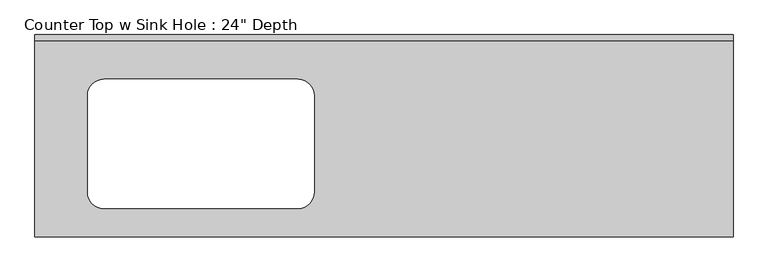
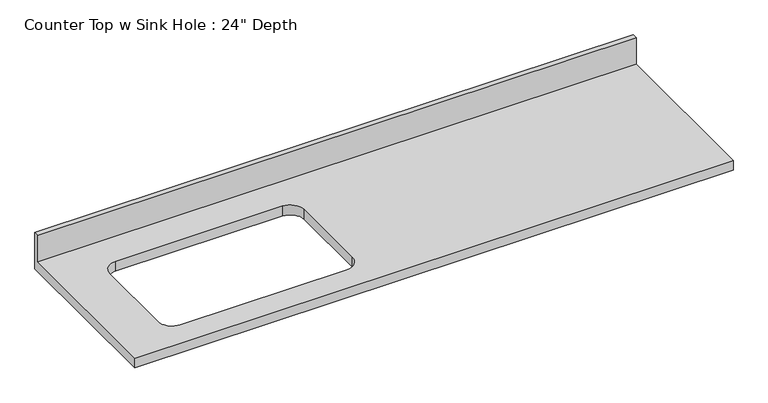
"""IFC4 building model written with IfcOpenShell, lengths in millimetres: furniture geometry."""

from ifc_helpers import new_model, si_unit, frame, origin, place, context, project, spatial, polyline, circle_curve, source, transform, mapped, element, save
from ifc_brep_helpers import plane_surface, revolved_surface, advanced_brep


def furniture_74614b7d(model_context):
    return source(origin(), model_context, "Body", "AdvancedBrep", [
        advanced_brep(
        [(-1200.4622951, -635.0, 914.4), (990.2877049, -635.0, 914.4), (990.2877049, -19.05, 914.4), (-1200.4622951, -19.05, 914.4), (-984.5622951, -139.7, 914.4), (-374.9622951, -139.7, 914.4), (-324.1622951, -190.5, 914.4), (-324.1622951, -495.3, 914.4), (-374.9622951, -546.1, 914.4), (-984.5622951, -546.1, 914.4), (-1035.3622951, -495.3, 914.4), (-1035.3622951, -190.5, 914.4), (990.2877049, 0.0, 876.3), (990.2877049, -635.0, 876.3), (-1200.4622951, -635.0, 876.3), (-1200.4622951, 0.0, 876.3), (-374.9622951, -139.7, 876.3), (-984.5622951, -139.7, 876.3), (-1035.3622951, -190.5, 876.3), (-1035.3622951, -495.3, 876.3), (-984.5622951, -546.1, 876.3), (-374.9622951, -546.1, 876.3), (-324.1622951, -495.3, 876.3), (-324.1622951, -190.5, 876.3), (-1200.4622951, 0.0, 1016.0), (990.2877049, 0.0, 1016.0), (-1200.4622951, -19.05, 1016.0), (990.2877049, -19.05, 1016.0)],
        [
            (0, 1),
            (1, 2),
            (2, 3),
            (3, 0),
            (4, 5),
            (5, 6, circle_curve(frame((-374.9622951, -190.5, 914.4), z_axis=(0.0, 0.0, -1.0), x_axis=(1.0, 0.0, 0.0)), 50.8)),
            (6, 7),
            (7, 8, circle_curve(frame((-374.9622951, -495.3, 914.4), z_axis=(0.0, 0.0, -1.0), x_axis=(1.0, 0.0, 0.0)), 50.8)),
            (8, 9),
            (9, 10, circle_curve(frame((-984.5622951, -495.3, 914.4), z_axis=(0.0, 0.0, -1.0), x_axis=(1.0, 0.0, 0.0)), 50.8)),
            (10, 11),
            (11, 4, circle_curve(frame((-984.5622951, -190.5, 914.4), z_axis=(0.0, 0.0, -1.0), x_axis=(1.0, 0.0, 0.0)), 50.8)),
            (12, 13),
            (13, 14),
            (14, 15),
            (15, 12),
            (16, 17),
            (17, 18, circle_curve(frame((-984.5622951, -190.5, 876.3), z_axis=(0.0, 0.0, 1.0), x_axis=(1.0, 0.0, 0.0)), 50.8)),
            (18, 19),
            (19, 20, circle_curve(frame((-984.5622951, -495.3, 876.3), z_axis=(0.0, 0.0, 1.0), x_axis=(1.0, 0.0, 0.0)), 50.8)),
            (20, 21),
            (21, 22, circle_curve(frame((-374.9622951, -495.3, 876.3), z_axis=(0.0, 0.0, 1.0), x_axis=(1.0, 0.0, 0.0)), 50.8)),
            (22, 23),
            (23, 16, circle_curve(frame((-374.9622951, -190.5, 876.3), z_axis=(0.0, 0.0, 1.0), x_axis=(1.0, 0.0, 0.0)), 50.8)),
            (15, 24),
            (24, 25),
            (25, 12),
            (14, 0),
            (3, 26),
            (26, 24),
            (13, 1),
            (25, 27),
            (27, 2),
            (26, 27),
            (4, 17),
            (16, 5),
            (11, 18),
            (10, 19),
            (9, 20),
            (8, 21),
            (7, 22),
            (6, 23),
        ],
        [
            plane_surface(frame((-1200.4622951, 0.0, 914.4), z_axis=(0.0, 0.0, 1.0), x_axis=(-1.0, 0.0, 0.0))),
            plane_surface(frame((-1200.4622951, 0.0, 876.3), z_axis=(0.0, 0.0, -1.0), x_axis=(1.0, 0.0, 0.0))),
            plane_surface(frame((990.2877049, 0.0, 914.4), z_axis=(0.0, 1.0, 0.0), x_axis=(0.0, 0.0, -1.0))),
            plane_surface(frame((-1200.4622951, 0.0, 914.4), z_axis=(-1.0, 0.0, 0.0), x_axis=(0.0, 0.0, -1.0))),
            plane_surface(frame((-1200.4622951, -635.0, 914.4), z_axis=(0.0, -1.0, 0.0), x_axis=(0.0, 0.0, -1.0))),
            plane_surface(frame((990.2877049, -635.0, 914.4), z_axis=(1.0, 0.0, 0.0), x_axis=(0.0, 0.0, -1.0))),
            plane_surface(frame((-1200.4622951, 0.0, 1016.0), z_axis=(0.0, 0.0, 1.0), x_axis=(0.0, -1.0, 0.0))),
            plane_surface(frame((-1200.4622951, -19.05, 1016.0), z_axis=(0.0, -1.0, 0.0), x_axis=(0.0, 0.0, -1.0))),
            plane_surface(frame((-374.9622951, -139.7, 914.4), z_axis=(0.0, -1.0, 0.0), x_axis=(0.0, 0.0, -1.0))),
            revolved_surface(polyline([(-933.7622951000001, -190.5, 914.4), (-933.7622951000001, -190.5, 876.3)]), (-984.5622951, -190.5, 876.3), (0.0, 0.0, 1.0)),
            plane_surface(frame((-1035.3622951, -190.5, 914.4), z_axis=(1.0, 0.0, 0.0), x_axis=(0.0, 0.0, -1.0))),
            revolved_surface(polyline([(-933.7622951000001, -495.3, 914.4), (-933.7622951000001, -495.3, 876.3)]), (-984.5622951, -495.3, 876.3), (0.0, 0.0, 1.0)),
            plane_surface(frame((-984.5622951, -546.1, 914.4), z_axis=(0.0, 1.0, 0.0), x_axis=(0.0, 0.0, -1.0))),
            revolved_surface(polyline([(-324.1622951, -495.3, 914.4), (-324.1622951, -495.3, 876.3)]), (-374.9622951, -495.3, 876.3), (0.0, 0.0, 1.0)),
            plane_surface(frame((-324.1622951, -495.3, 914.4), z_axis=(-1.0, 0.0, 0.0), x_axis=(0.0, 0.0, -1.0))),
            revolved_surface(polyline([(-324.1622951, -190.5, 914.4), (-324.1622951, -190.5, 876.3)]), (-374.9622951, -190.5, 876.3), (0.0, 0.0, 1.0)),
        ],
        [
            (0, [[1, 2, 3, 4], [5, 6, 7, 8, 9, 10, 11, 12]]),
            (1, [[13, 14, 15, 16], [17, 18, 19, 20, 21, 22, 23, 24]]),
            (2, [[-16, 25, 26, 27]]),
            (3, [[-15, 28, -4, 29, 30, -25]]),
            (4, [[-1, -28, -14, 31]]),
            (5, [[-13, -27, 32, 33, -2, -31]]),
            (6, [[-30, 34, -32, -26]]),
            (7, [[-34, -29, -3, -33]]),
            (8, [[35, -17, 36, -5]]),
            (9, [[-35, -12, 37, -18]]),
            (10, [[-37, -11, 38, -19]]),
            (11, [[-38, -10, 39, -20]]),
            (12, [[-39, -9, 40, -21]]),
            (13, [[-40, -8, 41, -22]]),
            (14, [[-41, -7, 42, -23]]),
            (15, [[-36, -24, -42, -6]]),
        ],
    ),
    ])


if __name__ == "__main__":
    model = new_model("IFC4")
    model_context = context("Model", 3, world=origin())
    ifc_project = project(units=[si_unit("LENGTHUNIT", "METRE", prefix="MILLI")], contexts=[model_context])
    site = spatial("IfcSite", under=ifc_project)
    building = spatial("IfcBuilding", under=site)
    placement = place(None, origin())
    furniture_shape = furniture_74614b7d(model_context)
    element("IfcFurniture", 1, ObjectType="Counter Top w Sink Hole : 24\" Depth", at=placement, inside=building, context=model_context, shape_type="MappedRepresentation", body=[
        mapped(furniture_shape, transform((0.0, 0.0, 0.0), x_axis=(1.0, 0.0, 0.0), y_axis=(0.0, 1.0, 0.0), z_axis=(0.0, 0.0, 1.0))),
    ])
    save(model, "model.ifc")

# Revit data of these elements
# Type "Counter Top w Sink Hole : 24\" Depth"
#   Assembly Code = "C1030400"
#   Counter Thickness = 0' - 1 1/2"
#   Depth = 2' - 1"
#   Height = 3' - 0"
#   Length [instance default] = 8' - 0"
#   Sink Location [instance default] = 2' - 0"
#   Sink Location To Wall [instance default] = 0' - 6"
#   Sink Opening Depth [instance default] = 1' - 3"
#   Sink Opening Width [instance default] = 2' - 3"
#   Counter Top Material = none
#   Default Elevation = 0
# Element 1 (IfcFurniture, "Counter Top w Sink Hole : 24\" Depth")
#   Length = 7' - 2 1/4"
#   Sink Location = 1' - 8 1/2"
#   Materials on its faces: "Counter Top"
# Materials
#   "Counter Top": class "Wood", colour RGB 226 177 128, transparency 0
